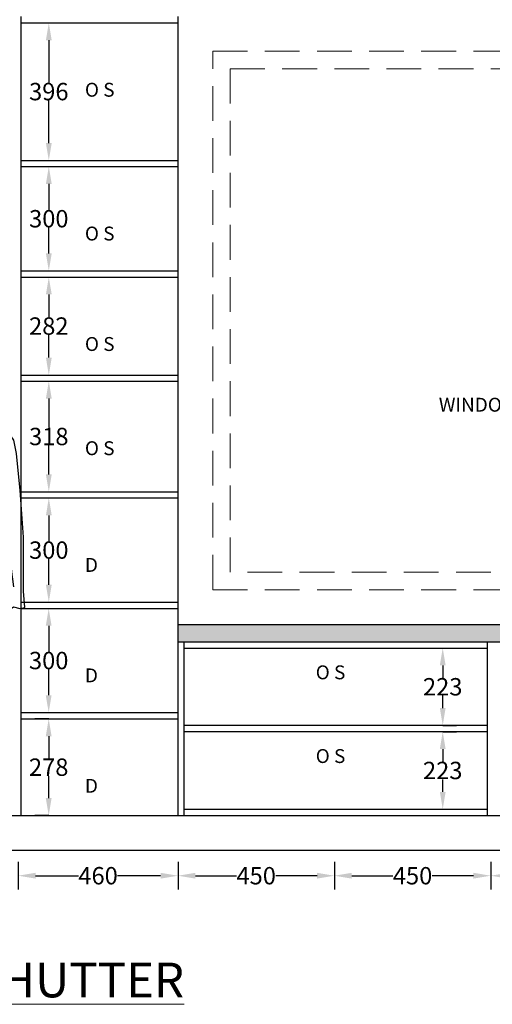
# Model space of a CAD drawing. Units: millimetres. Extents: x -472 to 16192, y -4730 to 4331.
# Tile 6 of 8: x 12774 to 14134, y -4730 to -1895. Entities that reach past the tile are written whole.
import ezdxf

# ---------------------------------------------------------------- set-up
doc = ezdxf.new("R2010")
doc.units = ezdxf.units.MM
doc.header["$MEASUREMENT"] = 0
doc.linetypes.add('DASHED', pattern=[0.75, 0.5, -0.25])
for name, color, linetype, lineweight in [('A-ANNO-DIMS', 2, 'Continuous', 18), ('A-ANNO-TEXT', 6, 'Continuous', 18), ('A-ELEV', 7, 'Continuous', 25), ('A-FURN', 8, 'Continuous', 25), ('A-GLAZ', 4, 'DASHED', 18)]:
    doc.layers.add(name, color=color, linetype=linetype, lineweight=lineweight)
doc.styles.get("Standard").update_dxf_attribs({"font": 'arial.ttf'})
doc.dimstyles.get("Standard").update_dxf_attribs({"dimtxt": 50, "dimasz": 50, "dimexe": 40, "dimexo": 40, "dimgap": 0.09, "dimtad": 0, "dimtih": 1, "dimtoh": 1, "dimdec": 0, "dimzin": 0, "dimdsep": 46, "dimtxsty": 'Standard', "dimcen": 0.09, "dimclrd": 1, "dimclre": 3, "dimclrt": 6, "dimadec": 0, "dimazin": 0, "dimtfac": 1, "dimtdec": 0, "dimtofl": 0, "dimtmove": 0, "dimatfit": 3, "dimfxl": 40, "dimfxlon": 1, "dimtolj": 1, "dimtzin": 0, "dimarcsym": 0})

# ---------------------------------------------------------------- blocks, each defined once
blk = doc.blocks.new('*D58')
at = {"layer": 'A-ANNO-DIMS', "color": 0, "lineweight": -2, "transparency": 16777216}
for p, q in [((12769.7, -4319.4), (12769.7, -4399.4)), ((13229.7, -4319.4), (13229.7, -4399.4)), ((12819.7, -4359.4), (12943.4, -4359.4)), ((13179.7, -4359.4), (13055.9, -4359.4))]:
    blk.add_line(p, q, dxfattribs=at)
at = {"layer": 'A-ANNO-DIMS', "color": 0, "transparency": 16777216}
for points in [[(12819.7, -4351), (12819.7, -4367.7), (12769.7, -4359.4)], [(13179.7, -4351), (13179.7, -4367.7), (13229.7, -4359.4)]]:
    blk.add_solid(points, dxfattribs=at)
at = {"layer": 'Defpoints', "color": 0, "transparency": 16777216}
for p in [(12769.7, -4185.9), (13229.7, -4185.9), (13229.7, -4359.4)]:
    blk.add_point(p, dxfattribs=at)
at = {"layer": 'A-ANNO-DIMS', "color": 0, "transparency": 16777216, "insert": (12999.7, -4359.4), "char_height": 50, "attachment_point": 5}
blk.add_mtext('\\A1;460', dxfattribs=at)
blk = doc.blocks.new('*D59')
at = {"layer": 'A-ANNO-DIMS', "color": 0, "lineweight": -2, "transparency": 16777216}
for p, q in [((13229.7, -4319.4), (13229.7, -4399.4)), ((13679.7, -4319.4), (13679.7, -4399.4)), ((13279.7, -4359.4), (13398.4, -4359.4)), ((13629.7, -4359.4), (13510.9, -4359.4))]:
    blk.add_line(p, q, dxfattribs=at)
at = {"layer": 'A-ANNO-DIMS', "color": 0, "transparency": 16777216}
for points in [[(13279.7, -4351), (13279.7, -4367.7), (13229.7, -4359.4)], [(13629.7, -4351), (13629.7, -4367.7), (13679.7, -4359.4)]]:
    blk.add_solid(points, dxfattribs=at)
at = {"layer": 'Defpoints', "color": 0, "transparency": 16777216}
for p in [(13229.7, -4185.9), (13679.7, -4185.9), (13679.7, -4359.4)]:
    blk.add_point(p, dxfattribs=at)
at = {"layer": 'A-ANNO-DIMS', "color": 0, "transparency": 16777216, "insert": (13454.7, -4359.4), "char_height": 50, "attachment_point": 5}
blk.add_mtext('\\A1;450', dxfattribs=at)
blk = doc.blocks.new('*D60')
at = {"layer": 'A-ANNO-DIMS', "color": 0, "lineweight": -2, "transparency": 16777216}
for p, q in [((13679.7, -4319.4), (13679.7, -4399.4)), ((14129.7, -4319.4), (14129.7, -4399.4)), ((13729.7, -4359.4), (13848.4, -4359.4)), ((14079.7, -4359.4), (13960.9, -4359.4))]:
    blk.add_line(p, q, dxfattribs=at)
at = {"layer": 'A-ANNO-DIMS', "color": 0, "transparency": 16777216}
for points in [[(13729.7, -4351), (13729.7, -4367.7), (13679.7, -4359.4)], [(14079.7, -4351), (14079.7, -4367.7), (14129.7, -4359.4)]]:
    blk.add_solid(points, dxfattribs=at)
at = {"layer": 'Defpoints', "color": 0, "transparency": 16777216}
for p in [(13679.7, -4185.9), (14129.7, -4185.9), (14129.7, -4359.4)]:
    blk.add_point(p, dxfattribs=at)
at = {"layer": 'A-ANNO-DIMS', "color": 0, "transparency": 16777216, "insert": (13904.7, -4359.4), "char_height": 50, "attachment_point": 5}
blk.add_mtext('\\A1;450', dxfattribs=at)
blk = doc.blocks.new('*D61')
at = {"layer": 'A-ANNO-DIMS', "color": 0, "lineweight": -2, "transparency": 16777216}
for p, q in [((14129.7, -4319.4), (14129.7, -4399.4)), ((14579.7, -4319.4), (14579.7, -4399.4)), ((14179.7, -4359.4), (14298.4, -4359.4)), ((14529.7, -4359.4), (14410.9, -4359.4))]:
    blk.add_line(p, q, dxfattribs=at)
at = {"layer": 'A-ANNO-DIMS', "color": 0, "transparency": 16777216}
for points in [[(14179.7, -4351), (14179.7, -4367.7), (14129.7, -4359.4)], [(14529.7, -4351), (14529.7, -4367.7), (14579.7, -4359.4)]]:
    blk.add_solid(points, dxfattribs=at)
at = {"layer": 'Defpoints', "color": 0, "transparency": 16777216}
for p in [(14129.7, -4185.9), (14579.7, -4185.9), (14579.7, -4359.4)]:
    blk.add_point(p, dxfattribs=at)
at = {"layer": 'A-ANNO-DIMS', "color": 0, "transparency": 16777216, "insert": (14354.7, -4359.4), "char_height": 50, "attachment_point": 5}
blk.add_mtext('\\A1;450', dxfattribs=at)
blk = doc.blocks.new('*D75')
at = {"layer": 'A-ANNO-DIMS', "color": 0, "lineweight": -2, "transparency": 16777216}
for p, q in [((12857.6, -3907.9), (12817.6, -3907.9)), ((12857.6, -3957.9), (12857.6, -4021.3)), ((12857.6, -4135.9), (12857.6, -4072.5)), ((12857.6, -4185.9), (12817.6, -4185.9))]:
    blk.add_line(p, q, dxfattribs=at)
at = {"layer": 'A-ANNO-DIMS', "color": 0, "transparency": 16777216}
for points in [[(12849.2, -3957.9), (12865.9, -3957.9), (12857.6, -3907.9)], [(12849.2, -4135.9), (12865.9, -4135.9), (12857.6, -4185.9)]]:
    blk.add_solid(points, dxfattribs=at)
at = {"layer": 'Defpoints', "color": 0, "transparency": 16777216}
for p in [(12857.6, -3907.9), (12886.2, -3907.9), (12886.2, -4185.9)]:
    blk.add_point(p, dxfattribs=at)
at = {"layer": 'A-ANNO-DIMS', "color": 0, "transparency": 16777216, "insert": (12857.6, -4046.9), "char_height": 50, "attachment_point": 5}
blk.add_mtext('\\A1;278', dxfattribs=at)
blk = doc.blocks.new('*D76')
at = {"layer": 'A-ANNO-DIMS', "color": 0, "lineweight": -2, "transparency": 16777216}
for p, q in [((12857.6, -3589.9), (12897.6, -3589.9)), ((12857.6, -3639.9), (12857.6, -3714.3)), ((12857.6, -3839.9), (12857.6, -3765.5)), ((12857.6, -3889.9), (12897.6, -3889.9))]:
    blk.add_line(p, q, dxfattribs=at)
at = {"layer": 'A-ANNO-DIMS', "color": 0, "transparency": 16777216}
for points in [[(12849.2, -3639.9), (12865.9, -3639.9), (12857.6, -3589.9)], [(12849.2, -3839.9), (12865.9, -3839.9), (12857.6, -3889.9)]]:
    blk.add_solid(points, dxfattribs=at)
at = {"layer": 'Defpoints', "color": 0, "transparency": 16777216}
for p in [(12857.6, -3589.9), (12857.6, -3589.9), (12857.6, -3889.9)]:
    blk.add_point(p, dxfattribs=at)
at = {"layer": 'A-ANNO-DIMS', "color": 0, "transparency": 16777216, "insert": (12857.6, -3739.9), "char_height": 50, "attachment_point": 5}
blk.add_mtext('\\A1;300', dxfattribs=at)
blk = doc.blocks.new('*D77')
at = {"layer": 'A-ANNO-DIMS', "color": 0, "lineweight": -2, "transparency": 16777216}
for p, q in [((12857.9, -3271.9), (12897.9, -3271.9)), ((12857.9, -3321.9), (12857.9, -3396.3)), ((12857.9, -3521.9), (12857.9, -3447.5)), ((12857.9, -3571.9), (12897.9, -3571.9))]:
    blk.add_line(p, q, dxfattribs=at)
at = {"layer": 'A-ANNO-DIMS', "color": 0, "transparency": 16777216}
for points in [[(12849.6, -3321.9), (12866.3, -3321.9), (12857.9, -3271.9)], [(12849.6, -3521.9), (12866.3, -3521.9), (12857.9, -3571.9)]]:
    blk.add_solid(points, dxfattribs=at)
at = {"layer": 'Defpoints', "color": 0, "transparency": 16777216}
for p in [(12857.9, -3271.9), (12857.9, -3271.9), (12857.9, -3571.9)]:
    blk.add_point(p, dxfattribs=at)
at = {"layer": 'A-ANNO-DIMS', "color": 0, "transparency": 16777216, "insert": (12857.9, -3421.9), "char_height": 50, "attachment_point": 5}
blk.add_mtext('\\A1;300', dxfattribs=at)
blk = doc.blocks.new('*D78')
at = {"layer": 'A-ANNO-DIMS', "color": 0, "lineweight": -2, "transparency": 16777216}
for p, q in [((12857.9, -2935.9), (12897.9, -2935.9)), ((12857.9, -2985.9), (12857.9, -3069.3)), ((12857.9, -3203.9), (12857.9, -3120.5)), ((12857.9, -3253.9), (12897.9, -3253.9))]:
    blk.add_line(p, q, dxfattribs=at)
at = {"layer": 'A-ANNO-DIMS', "color": 0, "transparency": 16777216}
for points in [[(12849.6, -2985.9), (12866.3, -2985.9), (12857.9, -2935.9)], [(12849.6, -3203.9), (12866.3, -3203.9), (12857.9, -3253.9)]]:
    blk.add_solid(points, dxfattribs=at)
at = {"layer": 'Defpoints', "color": 0, "transparency": 16777216}
for p in [(12857.9, -2935.9), (12857.9, -2935.9), (12857.9, -3253.9)]:
    blk.add_point(p, dxfattribs=at)
at = {"layer": 'A-ANNO-DIMS', "color": 0, "transparency": 16777216, "insert": (12857.9, -3094.9), "char_height": 50, "attachment_point": 5}
blk.add_mtext('\\A1;318', dxfattribs=at)
blk = doc.blocks.new('*D79')
at = {"layer": 'A-ANNO-DIMS', "color": 0, "lineweight": -2, "transparency": 16777216}
for p, q in [((12857.9, -2635.9), (12897.9, -2635.9)), ((12857.9, -2685.9), (12857.9, -2751.3)), ((12857.9, -2867.9), (12857.9, -2802.5)), ((12857.9, -2917.9), (12897.9, -2917.9))]:
    blk.add_line(p, q, dxfattribs=at)
at = {"layer": 'A-ANNO-DIMS', "color": 0, "transparency": 16777216}
for points in [[(12849.6, -2685.9), (12866.3, -2685.9), (12857.9, -2635.9)], [(12849.6, -2867.9), (12866.3, -2867.9), (12857.9, -2917.9)]]:
    blk.add_solid(points, dxfattribs=at)
at = {"layer": 'Defpoints', "color": 0, "transparency": 16777216}
for p in [(12857.9, -2635.9), (12857.9, -2635.9), (12857.9, -2917.9)]:
    blk.add_point(p, dxfattribs=at)
at = {"layer": 'A-ANNO-DIMS', "color": 0, "transparency": 16777216, "insert": (12857.9, -2776.9), "char_height": 50, "attachment_point": 5}
blk.add_mtext('\\A1;282', dxfattribs=at)
blk = doc.blocks.new('*D80')
at = {"layer": 'A-ANNO-DIMS', "color": 0, "lineweight": -2, "transparency": 16777216}
for p, q in [((12857.9, -2317.9), (12897.9, -2317.9)), ((12857.9, -2367.9), (12857.9, -2442.3)), ((12857.9, -2567.9), (12857.9, -2493.5)), ((12857.9, -2617.9), (12897.9, -2617.9))]:
    blk.add_line(p, q, dxfattribs=at)
at = {"layer": 'A-ANNO-DIMS', "color": 0, "transparency": 16777216}
for points in [[(12849.6, -2367.9), (12866.3, -2367.9), (12857.9, -2317.9)], [(12849.6, -2567.9), (12866.3, -2567.9), (12857.9, -2617.9)]]:
    blk.add_solid(points, dxfattribs=at)
at = {"layer": 'Defpoints', "color": 0, "transparency": 16777216}
for p in [(12857.9, -2317.9), (12857.9, -2317.9), (12857.9, -2617.9)]:
    blk.add_point(p, dxfattribs=at)
at = {"layer": 'A-ANNO-DIMS', "color": 0, "transparency": 16777216, "insert": (12857.9, -2467.9), "char_height": 50, "attachment_point": 5}
blk.add_mtext('\\A1;300', dxfattribs=at)
blk = doc.blocks.new('*D81')
at = {"layer": 'A-ANNO-DIMS', "color": 0, "lineweight": -2, "transparency": 16777216}
for p, q in [((12857.9, -1903.9), (12897.9, -1903.9)), ((12857.9, -1953.9), (12857.9, -2076.3)), ((12857.9, -2249.9), (12857.9, -2127.5)), ((12857.9, -2299.9), (12897.9, -2299.9))]:
    blk.add_line(p, q, dxfattribs=at)
at = {"layer": 'A-ANNO-DIMS', "color": 0, "transparency": 16777216}
for points in [[(12849.6, -1953.9), (12866.3, -1953.9), (12857.9, -1903.9)], [(12849.6, -2249.9), (12866.3, -2249.9), (12857.9, -2299.9)]]:
    blk.add_solid(points, dxfattribs=at)
at = {"layer": 'Defpoints', "color": 0, "transparency": 16777216}
for p in [(12857.9, -1903.9), (12857.9, -1903.9), (12857.9, -2299.9)]:
    blk.add_point(p, dxfattribs=at)
at = {"layer": 'A-ANNO-DIMS', "color": 0, "transparency": 16777216, "insert": (12857.9, -2101.9), "char_height": 50, "attachment_point": 5}
blk.add_mtext('\\A1;396', dxfattribs=at)
blk = doc.blocks.new('*D86')
at = {"layer": 'A-ANNO-DIMS', "color": 0, "lineweight": -2, "transparency": 16777216}
for p, q in [((11734.7, -2935.9), (11774.7, -2935.9)), ((11734.7, -2985.9), (11734.7, -3526.3)), ((11734.7, -4117.9), (11734.7, -3577.5)), ((11774.7, -4167.9), (11694.7, -4167.9))]:
    blk.add_line(p, q, dxfattribs=at)
at = {"layer": 'A-ANNO-DIMS', "color": 0, "transparency": 16777216}
for points in [[(11726.4, -2985.9), (11743, -2985.9), (11734.7, -2935.9)], [(11726.4, -4117.9), (11743, -4117.9), (11734.7, -4167.9)]]:
    blk.add_solid(points, dxfattribs=at)
at = {"layer": 'Defpoints', "color": 0, "transparency": 16777216}
for p in [(11734.7, -2935.9), (11734.7, -4167.9), (14004.4, -4167.9)]:
    blk.add_point(p, dxfattribs=at)
at = {"layer": 'A-ANNO-DIMS', "color": 0, "transparency": 16777216, "insert": (11734.7, -3551.9), "char_height": 50, "attachment_point": 5}
blk.add_mtext('\\A1;1232', dxfattribs=at)
blk = doc.blocks.new('*D87')
at = {"layer": 'A-ANNO-DIMS', "color": 0, "lineweight": -2, "transparency": 16777216}
for p, q in [((11774.7, -3944.9), (11694.7, -3944.9)), ((11734.7, -3994.9), (11734.7, -4030.8)), ((11734.7, -4117.9), (11734.7, -4082)), ((11774.7, -4167.9), (11694.7, -4167.9))]:
    blk.add_line(p, q, dxfattribs=at)
at = {"layer": 'A-ANNO-DIMS', "color": 0, "transparency": 16777216}
for points in [[(11726.4, -3994.9), (11743, -3994.9), (11734.7, -3944.9)], [(11726.4, -4117.9), (11743, -4117.9), (11734.7, -4167.9)]]:
    blk.add_solid(points, dxfattribs=at)
at = {"layer": 'Defpoints', "color": 0, "transparency": 16777216}
for p in [(11734.7, -3944.9), (13999.1, -3944.9), (14004.4, -4167.9)]:
    blk.add_point(p, dxfattribs=at)
at = {"layer": 'A-ANNO-DIMS', "color": 0, "transparency": 16777216, "insert": (11734.7, -4056.4), "char_height": 50, "attachment_point": 5}
blk.add_mtext('\\A1;223', dxfattribs=at)
blk = doc.blocks.new('*D88')
at = {"layer": 'A-ANNO-DIMS', "color": 0, "lineweight": -2, "transparency": 16777216}
for p, q in [((13991.5, -3944.9), (14031.5, -3944.9)), ((13991.5, -3994.9), (13991.5, -4030.8)), ((13991.5, -4117.9), (13991.5, -4082)), ((13991.5, -4167.9), (14031.5, -4167.9))]:
    blk.add_line(p, q, dxfattribs=at)
at = {"layer": 'A-ANNO-DIMS', "color": 0, "transparency": 16777216}
for points in [[(13983.2, -3994.9), (13999.8, -3994.9), (13991.5, -3944.9)], [(13983.2, -4117.9), (13999.8, -4117.9), (13991.5, -4167.9)]]:
    blk.add_solid(points, dxfattribs=at)
at = {"layer": 'Defpoints', "color": 0, "transparency": 16777216}
for p in [(13973.3, -3944.9), (13991.5, -3944.9), (13973.3, -4167.9)]:
    blk.add_point(p, dxfattribs=at)
at = {"layer": 'A-ANNO-DIMS', "color": 0, "transparency": 16777216, "insert": (13991.5, -4056.4), "char_height": 50, "attachment_point": 5}
blk.add_mtext('\\A1;223', dxfattribs=at)
blk = doc.blocks.new('*D89')
at = {"layer": 'A-ANNO-DIMS', "color": 0, "lineweight": -2, "transparency": 16777216}
for p, q in [((13991.5, -3703.9), (14031.5, -3703.9)), ((13991.5, -3753.9), (13991.5, -3789.8)), ((13991.5, -3876.9), (13991.5, -3841)), ((13991.5, -3926.9), (14031.5, -3926.9))]:
    blk.add_line(p, q, dxfattribs=at)
at = {"layer": 'A-ANNO-DIMS', "color": 0, "transparency": 16777216}
for points in [[(13983.2, -3753.9), (13999.8, -3753.9), (13991.5, -3703.9)], [(13983.2, -3876.9), (13999.8, -3876.9), (13991.5, -3926.9)]]:
    blk.add_solid(points, dxfattribs=at)
at = {"layer": 'Defpoints', "color": 0, "transparency": 16777216}
for p in [(13991.5, -3703.9), (13991.5, -3703.9), (13991.5, -3926.9)]:
    blk.add_point(p, dxfattribs=at)
at = {"layer": 'A-ANNO-DIMS', "color": 0, "transparency": 16777216, "insert": (13991.5, -3815.4), "char_height": 50, "attachment_point": 5}
blk.add_mtext('\\A1;223', dxfattribs=at)
blk = doc.blocks.new('7')
for p, q in [((3901.77, 12903.37), (3898.37, 12903.37)), ((3898.37, 12903.37), (3898.37, 12902.56)), ((3901.6, 12902.56), (3898.37, 12902.56)), ((3901.81, 12902.56), (3906.72, 12902.56)), ((3902.01, 12903.37), (3906.88, 12903.37)), ((3903.8, 12903.37), (3905.4, 12903.37)), ((3906.93, 12902.56), (3911.77, 12902.56)), ((3907.13, 12903.37), (3911.93, 12903.37)), ((3911.97, 12902.56), (3916.93, 12902.56)), ((3912.18, 12903.37), (3917.09, 12903.37)), ((3917.13, 12902.56), (3921.77, 12902.56)), ((3917.33, 12903.37), (3921.94, 12903.37)), ((3921.98, 12902.56), (3927.26, 12902.56)), ((3922.18, 12903.37), (3927.26, 12903.37)), ((3927.26, 12903.37), (3927.26, 12902.56)), ((3901.99, 12900.85), (3901.37, 12900)), ((3902.38, 12900.93), (3901.99, 12900.85)), ((3902.35, 12900.89), (3902.35, 12901.61)), ((3902.69, 12900.85), (3902.38, 12900.93)), ((3902.55, 12901.75), (3902.55, 12900.89)), ((3903.23, 12900.39), (3902.69, 12900.85)), ((3907.13, 12900.85), (3906.51, 12900)), ((3907.52, 12900.93), (3907.13, 12900.85)), ((3907.47, 12900.89), (3907.47, 12901.61)), ((3907.83, 12900.85), (3907.52, 12900.93)), ((3907.67, 12901.75), (3907.67, 12900.89)), ((3908.37, 12900.39), (3907.83, 12900.85)), ((3912.25, 12900.85), (3911.62, 12900)), ((3912.63, 12900.93), (3912.25, 12900.85)), ((3912.51, 12900.89), (3912.51, 12901.61)), ((3912.94, 12900.85), (3912.63, 12900.93)), ((3912.72, 12901.75), (3912.72, 12900.89)), ((3913.49, 12900.39), (3912.94, 12900.85)), ((3917.39, 12900.85), (3916.76, 12900)), ((3917.77, 12900.93), (3917.39, 12900.85)), ((3917.67, 12900.91), (3917.67, 12901.61)), ((3918.08, 12900.85), (3917.77, 12900.93)), ((3917.87, 12901.75), (3917.87, 12900.92)), ((3918.63, 12900.39), (3918.08, 12900.85)), ((3922.16, 12900.76), (3921.8, 12900.21)), ((3922.57, 12901.03), (3922.16, 12900.76)), ((3922.57, 12901.03), (3922.35, 12900.7)), ((3922.52, 12901), (3922.52, 12901.61)), ((3922.75, 12901), (3922.57, 12901.03)), ((3922.72, 12901.75), (3922.72, 12901.02)), ((3923.13, 12900.79), (3922.75, 12901)), ((3923.47, 12900.38), (3923.13, 12900.79)), ((3901.37, 12900), (3900.98, 12899.12)), ((3903.54, 12899.74), (3903.23, 12900.39)), ((3903.78, 12899.26), (3903.54, 12899.74)), ((3906.51, 12900), (3906.12, 12899.12)), ((3908.68, 12899.74), (3908.37, 12900.39)), ((3908.92, 12899.26), (3908.68, 12899.74)), ((3911.62, 12900), (3911.24, 12899.12)), ((3913.8, 12899.74), (3913.49, 12900.39)), ((3914.03, 12899.26), (3913.8, 12899.74)), ((3916.76, 12900), (3916.38, 12899.12)), ((3918.94, 12899.74), (3918.63, 12900.39)), ((3919.17, 12899.26), (3918.94, 12899.74)), ((3921.6, 12899.78), (3921.4, 12899.16)), ((3921.8, 12900.21), (3921.6, 12899.78)), ((3922.02, 12899.87), (3921.8, 12899.21)), ((3922.35, 12900.7), (3922.02, 12899.87)), ((3923.71, 12900.01), (3923.47, 12900.38)), ((3924, 12899.6), (3923.71, 12900.01)), ((3924.38, 12899.09), (3923.92, 12899.61)), ((3924, 12899.6), (3924.26, 12898.31)), ((3900.85, 12898.74), (3899.74, 12897.19)), ((3900.98, 12899.12), (3900.85, 12898.73)), ((3901.25, 12897.93), (3900.85, 12898.74)), ((3902.03, 12896.26), (3901.25, 12897.93)), ((3902.33, 12898.32), (3901.78, 12897.67)), ((3903.03, 12897.88), (3902.33, 12898.32)), ((3903.88, 12897.03), (3903.03, 12897.88)), ((3904.15, 12899.04), (3903.78, 12899.26)), ((3903.78, 12899.26), (3903.89, 12898.71)), ((3903.89, 12898.71), (3903.85, 12897.04)), ((3904.63, 12898.37), (3904.15, 12899.04)), ((3905.24, 12897.91), (3904.63, 12898.37)), ((3905.99, 12898.74), (3904.88, 12897.19)), ((3906.12, 12899.12), (3905.99, 12898.73)), ((3906.39, 12897.93), (3905.99, 12898.74)), ((3907.17, 12896.26), (3906.39, 12897.93)), ((3907.47, 12898.32), (3906.92, 12897.67)), ((3908.17, 12897.88), (3907.47, 12898.32)), ((3909.02, 12897.03), (3908.17, 12897.88)), ((3909.29, 12899.04), (3908.92, 12899.26)), ((3908.92, 12899.26), (3909.03, 12898.71)), ((3909.03, 12898.71), (3908.99, 12897.04)), ((3909.77, 12898.37), (3909.29, 12899.04)), ((3910.38, 12897.91), (3909.77, 12898.37)), ((3911.1, 12898.74), (3909.99, 12897.19)), ((3911.51, 12897.93), (3911.1, 12898.74)), ((3911.24, 12899.12), (3911.11, 12898.73)), ((3912.29, 12896.26), (3911.51, 12897.93)), ((3912.58, 12898.32), (3912.04, 12897.67)), ((3913.28, 12897.88), (3912.58, 12898.32)), ((3914.13, 12897.03), (3913.28, 12897.88)), ((3914.4, 12899.04), (3914.03, 12899.26)), ((3914.03, 12899.26), (3914.14, 12898.71)), ((3914.14, 12898.71), (3914.11, 12897.04)), ((3914.88, 12898.37), (3914.4, 12899.04)), ((3915.5, 12897.91), (3914.88, 12898.37)), ((3916.24, 12898.74), (3915.13, 12897.19)), ((3916.65, 12897.93), (3916.24, 12898.74)), ((3916.38, 12899.12), (3916.25, 12898.73)), ((3917.43, 12896.26), (3916.65, 12897.93)), ((3917.72, 12898.32), (3917.18, 12897.67)), ((3918.42, 12897.88), (3917.72, 12898.32)), ((3919.27, 12897.03), (3918.42, 12897.88)), ((3919.54, 12899.04), (3919.17, 12899.26)), ((3919.17, 12899.26), (3919.28, 12898.71)), ((3919.28, 12898.71), (3919.25, 12897.04)), ((3920.02, 12898.37), (3919.54, 12899.04)), ((3920.64, 12897.91), (3920.02, 12898.37)), ((3920.43, 12897.51), (3920.79, 12898.19)), ((3920.79, 12898.19), (3921.19, 12898.97)), ((3921.19, 12898.97), (3921.35, 12899.23)), ((3921.3, 12899.16), (3921.61, 12898.57)), ((3921.35, 12899.23), (3921.7, 12898.97)), ((3921.61, 12898.57), (3922.15, 12897.07)), ((3921.66, 12898.64), (3921.65, 12898.56)), ((3921.8, 12899.21), (3921.66, 12898.64)), ((3921.7, 12898.97), (3921.75, 12898.95)), ((3922.33, 12897.95), (3922.18, 12897.46)), ((3922.55, 12898.4), (3922.33, 12897.95)), ((3922.82, 12898.65), (3922.55, 12898.4)), ((3923.17, 12898.44), (3922.82, 12898.65)), ((3923.96, 12897.86), (3923.17, 12898.44)), ((3924.26, 12898.31), (3924.56, 12897.43)), ((3925.4, 12898.1), (3924.38, 12899.09)), ((3925.37, 12898.1), (3926.22, 12897.58)), ((3925.98, 12896.74), (3925.4, 12898.1)), ((3899.74, 12897.04), (3896.88, 12894.08)), ((3900.49, 12895.54), (3899.68, 12897.02)), ((3899.74, 12897.19), (3899.74, 12897.04)), ((3901.78, 12897.67), (3901.59, 12897.2)), ((3904.88, 12897.04), (3902.02, 12894.08)), ((3903.85, 12897.04), (3903.46, 12895.81)), ((3905.63, 12895.54), (3904.82, 12897.02)), ((3904.88, 12897.19), (3904.88, 12897.04)), ((3906.92, 12897.67), (3906.73, 12897.2)), ((3909.99, 12897.04), (3907.14, 12894.08)), ((3908.99, 12897.04), (3908.6, 12895.81)), ((3910.75, 12895.54), (3909.93, 12897.02)), ((3909.99, 12897.19), (3909.99, 12897.04)), ((3912.04, 12897.67), (3911.85, 12897.2)), ((3915.13, 12897.04), (3912.28, 12894.08)), ((3914.11, 12897.04), (3913.72, 12895.81)), ((3915.89, 12895.54), (3915.07, 12897.02)), ((3915.13, 12897.19), (3915.13, 12897.04)), ((3917.18, 12897.67), (3916.99, 12897.2)), ((3918.8, 12895.75), (3920.32, 12897.13)), ((3919.25, 12897.04), (3918.86, 12895.81)), ((3920.32, 12897.13), (3920.43, 12897.51)), ((3921.88, 12892.78), (3920.35, 12897.12)), ((3922.18, 12897.46), (3922.13, 12897.29)), ((3922.15, 12897.07), (3923.16, 12894.25)), ((3924.48, 12897.51), (3923.96, 12897.86)), ((3924.56, 12897.43), (3925.04, 12890.79)), ((3926.43, 12894.14), (3925.98, 12896.74)), ((3926.22, 12897.58), (3927.16, 12897.19)), ((3927.16, 12897.19), (3927.49, 12896.83)), ((3927.49, 12896.83), (3928.42, 12895.42)), ((3901.42, 12893.5), (3900.49, 12895.54)), ((3902.61, 12894.93), (3902.03, 12896.26)), ((3906.56, 12893.5), (3905.63, 12895.54)), ((3907.75, 12894.93), (3907.17, 12896.26)), ((3911.68, 12893.5), (3910.75, 12895.54)), ((3912.86, 12894.93), (3912.29, 12896.26)), ((3916.82, 12893.5), (3915.89, 12895.54)), ((3916.93, 12893.82), (3918.8, 12895.75)), ((3918, 12894.93), (3917.43, 12896.26)), ((3928.42, 12895.42), (3928.82, 12893.49)), ((3896.88, 12894.08), (3896.21, 12893.3)), ((3902.02, 12894.08), (3901.35, 12893.3)), ((3907.14, 12894.08), (3906.47, 12893.3)), ((3912.28, 12894.08), (3911.61, 12893.3)), ((3916.66, 12893.06), (3916.93, 12893.82)), ((3923.16, 12894.25), (3924.99, 12889.48)), ((3926.01, 12893.3), (3926.43, 12894.14)), ((3896.21, 12893.3), (3895.68, 12890.13)), ((3901.35, 12893.3), (3900.82, 12890.13)), ((3906.47, 12893.3), (3905.93, 12890.13)), ((3911.61, 12893.3), (3911.07, 12890.13)), ((3916.38, 12890.58), (3916.66, 12893.06)), ((3922.78, 12892.51), (3921.88, 12892.78)), ((3922.52, 12890.85), (3922.78, 12892.51)), ((3926.86, 12892.12), (3926.01, 12893.3)), ((3928.82, 12893.49), (3929.34, 12888.11)), ((3925.72, 12886.84), (3922.52, 12890.85)), ((3925.04, 12890.79), (3925.04, 12889.46)), ((3925.8, 12887.26), (3926.86, 12892.12)), ((3895.68, 12890.13), (3894.93, 12877.55)), ((3900.82, 12890.13), (3900.07, 12877.55)), ((3905.93, 12890.13), (3905.19, 12877.55)), ((3911.07, 12890.13), (3910.33, 12877.55)), ((3916.04, 12887.47), (3916.38, 12890.58)), ((3924.99, 12889.48), (3926.22, 12885.93)), ((3899.96, 12887.35), (3900.04, 12889.01)), ((3905.1, 12887.35), (3905.18, 12889.01)), ((3910.22, 12887.35), (3910.29, 12889.01)), ((3915.36, 12887.35), (3915.43, 12889.01)), ((3920.32, 12887.26), (3920.4, 12888.92)), ((3929.34, 12888.11), (3929.84, 12881.39)), ((3899.6, 12883.53), (3899.96, 12887.35)), ((3904.74, 12883.53), (3905.1, 12887.35)), ((3909.86, 12883.53), (3910.22, 12887.35)), ((3915, 12883.53), (3915.36, 12887.35)), ((3915.76, 12883.2), (3916.04, 12887.47)), ((3919.96, 12883.44), (3920.32, 12887.26)), ((3926.26, 12885.67), (3925.72, 12886.84)), ((3926.3, 12885.33), (3926.19, 12876.54)), ((3926.22, 12885.93), (3926.3, 12885.33)), ((3899.17, 12879.56), (3899.6, 12883.53)), ((3904.31, 12879.56), (3904.74, 12883.53)), ((3909.43, 12879.56), (3909.86, 12883.53)), ((3914.57, 12879.56), (3915, 12883.53)), ((3915.21, 12878.72), (3915.76, 12883.2)), ((3919.53, 12879.47), (3919.96, 12883.44)), ((3929.84, 12881.39), (3929.84, 12873.56)), ((3898.52, 12873.79), (3899.17, 12879.56)), ((3903.66, 12873.79), (3904.31, 12879.56)), ((3908.78, 12873.79), (3909.43, 12879.56)), ((3913.92, 12873.79), (3914.57, 12879.56)), ((3918.88, 12873.7), (3919.53, 12879.47)), ((3915, 12874.51), (3915.21, 12878.72)), ((3894.93, 12877.55), (3894.8, 12871.54)), ((3900.07, 12877.55), (3899.94, 12871.54)), ((3905.19, 12877.55), (3905.06, 12871.54)), ((3910.33, 12877.55), (3910.2, 12871.54)), ((3926.19, 12876.54), (3925.98, 12872.58)), ((3898.24, 12871.2), (3898.52, 12873.79)), ((3903.38, 12871.2), (3903.66, 12873.79)), ((3908.49, 12871.2), (3908.78, 12873.79)), ((3913.63, 12871.2), (3913.92, 12873.79)), ((3914.56, 12870.79), (3915, 12874.51)), ((3918.52, 12870.38), (3918.88, 12873.7)), ((3925.98, 12872.58), (3925.91, 12870.44)), ((3929.84, 12873.56), (3930.02, 12871.22)), ((3895.48, 12871.28), (3894.8, 12871.54)), ((3897.11, 12871.35), (3895.48, 12871.28)), ((3899.2, 12871.07), (3897.11, 12871.35)), ((3900.62, 12871.28), (3899.94, 12871.54)), ((3902.25, 12871.35), (3900.62, 12871.28)), ((3904.34, 12871.07), (3902.25, 12871.35)), ((3905.74, 12871.28), (3905.06, 12871.54)), ((3907.37, 12871.35), (3905.74, 12871.28)), ((3909.45, 12871.07), (3907.37, 12871.35)), ((3910.88, 12871.28), (3910.2, 12871.54)), ((3912.51, 12871.35), (3910.88, 12871.28)), ((3914.59, 12871.07), (3912.51, 12871.35)), ((3927.43, 12870.57), (3928.42, 12871.3)), ((3928.42, 12871.3), (3929.35, 12871.09)), ((3929.35, 12871.09), (3930.07, 12871.23)), ((3915.15, 12870.57), (3914.56, 12870.79)), ((3916.78, 12870.64), (3915.15, 12870.57)), ((3918.41, 12870.42), (3916.78, 12870.64)), ((3918.56, 12870.49), (3923.07, 12869.98)), ((3923.07, 12869.98), (3925.95, 12870.34)), ((3925.95, 12870.34), (3927.43, 12870.57))]:
    blk.add_line(p, q)
for centre, radius, start, end in [((3902.79, 12902.74), 1.19, 31.4138, 165.4823), ((3902.79, 12902.74), 0.991, 38.898, 165.4823), ((3907.9, 12902.74), 1.19, 31.4138, 165.4823), ((3907.9, 12902.74), 0.991, 38.898, 165.4823), ((3912.95, 12902.74), 1.19, 31.4138, 165.4823), ((3912.95, 12902.74), 0.991, 38.898, 165.4823), ((3918.11, 12902.74), 1.19, 31.4138, 165.4823), ((3918.11, 12902.74), 0.991, 38.898, 165.4823), ((3922.95, 12902.74), 1.19, 31.4138, 165.4823), ((3922.95, 12902.74), 0.991, 38.898, 165.4823), ((3902.81, 12902.74), 1.22, 165.4823, 247.8669), ((3902.81, 12902.74), 1.02, 165.4823, 255.3823), ((3902.7, 12902.33), 0.991, 354.9774, 12.9498), ((3903.79, 12902.23), 0.102, 171.8983, 358.0565), ((3902.7, 12902.33), 1.19, 354.9774, 10.7201), ((3907.93, 12902.74), 1.22, 165.4823, 247.8669), ((3907.93, 12902.74), 1.02, 165.4823, 255.3823), ((3907.81, 12902.33), 0.991, 354.9774, 12.9498), ((3908.9, 12902.23), 0.102, 171.8983, 358.0565), ((3907.81, 12902.33), 1.19, 354.9774, 10.7201), ((3912.97, 12902.74), 1.22, 165.4823, 247.8669), ((3912.97, 12902.74), 1.02, 165.4823, 255.3823), ((3912.86, 12902.33), 0.991, 354.9774, 12.9498), ((3913.95, 12902.23), 0.102, 171.8983, 358.0565), ((3912.86, 12902.33), 1.19, 354.9774, 10.7201), ((3918.13, 12902.74), 1.22, 165.4823, 247.8669), ((3918.13, 12902.74), 1.02, 165.4823, 255.3823), ((3918.02, 12902.33), 0.991, 354.9774, 12.9498), ((3919.11, 12902.23), 0.102, 171.8983, 358.0565), ((3918.02, 12902.33), 1.19, 354.9774, 10.7201), ((3922.98, 12902.74), 1.22, 165.4823, 247.8669), ((3922.98, 12902.74), 1.02, 165.4823, 255.3823), ((3922.87, 12902.33), 0.991, 354.9774, 12.9498), ((3923.95, 12902.23), 0.102, 171.8983, 358.0565), ((3922.87, 12902.33), 1.19, 354.9774, 10.7201), ((3897.26, 12891.85), 1.97, 15.7523, 111.1565), ((3902.4, 12891.85), 1.97, 15.7523, 111.1565), ((3907.51, 12891.85), 1.97, 15.7523, 111.1565), ((3912.65, 12891.85), 1.97, 15.7523, 111.1565), ((3917.62, 12891.76), 1.97, 15.7523, 111.1565), ((3890.5, 12887.86), 9.47, 359.9116, 24.988), ((3895.64, 12887.86), 9.47, 359.9116, 24.988), ((3900.76, 12887.86), 9.47, 359.9116, 24.988), ((3905.9, 12887.86), 9.47, 359.9116, 24.988), ((3910.86, 12887.76), 9.47, 359.9116, 24.988), ((4029.55, 12886.77), 101.91, 177.2767, 187.0811), ((3861.53, 12885.02), 36.92, 343.5409, 5.9886), ((3866.67, 12885.02), 36.92, 343.5409, 5.9886), ((3876.93, 12885.02), 36.92, 343.5409, 5.9886), ((3881.89, 12884.93), 36.92, 343.5409, 5.9886)]:
    blk.add_arc(centre, radius, start, end)
for centre in [(3925.62, 12884.08), (3925.62, 12878.91), (3925.62, 12873.74)]:
    blk.add_ellipse(centre, major_axis=(0, 0.503), ratio=0.580645)
blk = doc.blocks.new('*D100')
at = {"layer": 'A-ANNO-DIMS', "color": 1, "lineweight": -2, "transparency": 16777216}
for p, q in [((16116.7, -1835.9), (16116.7, -1785.9)), ((16116.7, -2035.9), (16116.7, -2085.9))]:
    blk.add_line(p, q, dxfattribs=at)
at = {"layer": 'A-ANNO-DIMS', "color": 3, "lineweight": -2, "transparency": 16777216}
for p, q in [((16076.7, -1885.9), (16156.7, -1885.9)), ((16076.7, -1985.9), (16156.7, -1985.9))]:
    blk.add_line(p, q, dxfattribs=at)
at = {"layer": 'A-ANNO-DIMS', "color": 1, "transparency": 16777216}
for points in [[(16108.3, -1835.9), (16125, -1835.9), (16116.7, -1885.9)], [(16108.3, -2035.9), (16125, -2035.9), (16116.7, -1985.9)]]:
    blk.add_solid(points, dxfattribs=at)
at = {"layer": 'Defpoints', "color": 0, "transparency": 16777216}
for p in [(5309, -1885.9), (5209, -1985.9), (16116.7, -1985.9)]:
    blk.add_point(p, dxfattribs=at)
at = {"layer": 'A-ANNO-DIMS', "color": 6, "transparency": 16777216, "insert": (16116.7, -1935.9), "char_height": 50, "attachment_point": 5}
blk.add_mtext('\\A1;100', dxfattribs=at)
blk = doc.blocks.new('*D101')
at = {"layer": 'A-ANNO-DIMS', "color": 3, "lineweight": -2, "transparency": 16777216}
for p, q in [((16076.7, -1985.9), (16156.7, -1985.9)), ((16076.7, -3535.9), (16156.7, -3535.9))]:
    blk.add_line(p, q, dxfattribs=at)
at = {"layer": 'A-ANNO-DIMS', "color": 1, "lineweight": -2, "transparency": 16777216}
for p, q in [((16116.7, -2035.9), (16116.7, -2735.3)), ((16116.7, -3485.9), (16116.7, -2786.5))]:
    blk.add_line(p, q, dxfattribs=at)
at = {"layer": 'A-ANNO-DIMS', "color": 1, "transparency": 16777216}
for points in [[(16108.3, -2035.9), (16125, -2035.9), (16116.7, -1985.9)], [(16108.3, -3485.9), (16125, -3485.9), (16116.7, -3535.9)]]:
    blk.add_solid(points, dxfattribs=at)
at = {"layer": 'Defpoints', "color": 0, "transparency": 16777216}
for p in [(5209, -1985.9), (5209, -3535.9), (16116.7, -3535.9)]:
    blk.add_point(p, dxfattribs=at)
at = {"layer": 'A-ANNO-DIMS', "color": 6, "transparency": 16777216, "insert": (16116.7, -2760.9), "char_height": 50, "attachment_point": 5}
blk.add_mtext('\\A1;1550', dxfattribs=at)
blk = doc.blocks.new('*D102')
at = {"layer": 'A-ANNO-DIMS', "color": 3, "lineweight": -2, "transparency": 16777216}
for p, q in [((16076.7, -2035.9), (16156.7, -2035.9)), ((16076.7, -3485.9), (16156.7, -3485.9))]:
    blk.add_line(p, q, dxfattribs=at)
at = {"layer": 'A-ANNO-DIMS', "color": 1, "lineweight": -2, "transparency": 16777216}
for p, q in [((16116.7, -2085.9), (16116.7, -2735.3)), ((16116.7, -3435.9), (16116.7, -2786.5))]:
    blk.add_line(p, q, dxfattribs=at)
at = {"layer": 'A-ANNO-DIMS', "color": 1, "transparency": 16777216}
for points in [[(16108.3, -2085.9), (16125, -2085.9), (16116.7, -2035.9)], [(16108.3, -3435.9), (16125, -3435.9), (16116.7, -3485.9)]]:
    blk.add_solid(points, dxfattribs=at)
at = {"layer": 'Defpoints', "color": 0, "transparency": 16777216}
for p in [(5159, -2035.9), (5159, -3485.9), (16116.7, -3485.9)]:
    blk.add_point(p, dxfattribs=at)
at = {"layer": 'A-ANNO-DIMS', "color": 6, "transparency": 16777216, "insert": (16116.7, -2760.9), "char_height": 50, "attachment_point": 5}
blk.add_mtext('\\A1;1450', dxfattribs=at)
blk = doc.blocks.new('*D103')
at = {"layer": 'A-ANNO-DIMS', "color": 1, "lineweight": -2, "transparency": 16777216}
for p, q in [((16116.7, -3485.9), (16116.7, -3435.9)), ((16116.7, -3685.9), (16116.7, -3735.9))]:
    blk.add_line(p, q, dxfattribs=at)
at = {"layer": 'A-ANNO-DIMS', "color": 3, "lineweight": -2, "transparency": 16777216}
for p, q in [((16076.7, -3535.9), (16156.7, -3535.9)), ((16076.7, -3635.9), (16156.7, -3635.9))]:
    blk.add_line(p, q, dxfattribs=at)
at = {"layer": 'A-ANNO-DIMS', "color": 1, "transparency": 16777216}
for points in [[(16108.3, -3485.9), (16125, -3485.9), (16116.7, -3535.9)], [(16108.3, -3685.9), (16125, -3685.9), (16116.7, -3635.9)]]:
    blk.add_solid(points, dxfattribs=at)
at = {"layer": 'Defpoints', "color": 0, "transparency": 16777216}
for p in [(5209, -3535.9), (5309, -3635.9), (16116.7, -3635.9)]:
    blk.add_point(p, dxfattribs=at)
at = {"layer": 'A-ANNO-DIMS', "color": 6, "transparency": 16777216, "insert": (16116.7, -3585.9), "char_height": 50, "attachment_point": 5}
blk.add_mtext('\\A1;100', dxfattribs=at)
blk = doc.blocks.new('*D104')
at = {"layer": 'A-ANNO-DIMS', "color": 1, "lineweight": -2, "transparency": 16777216}
for p, q in [((16116.7, -3585.9), (16116.7, -3535.9)), ((16116.7, -3735.9), (16116.7, -3785.9)), ((16116.7, -3785.9), (16066.7, -3785.9))]:
    blk.add_line(p, q, dxfattribs=at)
at = {"layer": 'A-ANNO-DIMS', "color": 3, "lineweight": -2, "transparency": 16777216}
for p, q in [((16076.7, -3635.9), (16156.7, -3635.9)), ((16076.7, -3685.9), (16156.7, -3685.9))]:
    blk.add_line(p, q, dxfattribs=at)
at = {"layer": 'A-ANNO-DIMS', "color": 1, "transparency": 16777216}
for points in [[(16108.3, -3585.9), (16125, -3585.9), (16116.7, -3635.9)], [(16108.3, -3735.9), (16125, -3735.9), (16116.7, -3685.9)]]:
    blk.add_solid(points, dxfattribs=at)
at = {"layer": 'Defpoints', "color": 0, "transparency": 16777216}
for p in [(5309, -3635.9), (5309, -3685.9), (16116.7, -3685.9)]:
    blk.add_point(p, dxfattribs=at)
at = {"layer": 'A-ANNO-DIMS', "color": 6, "transparency": 16777216, "insert": (16030.8, -3785.9), "char_height": 50, "attachment_point": 5}
blk.add_mtext('\\A1;50', dxfattribs=at)
blk = doc.blocks.new('*D106')
at = {"layer": 'A-ANNO-DIMS', "color": 3, "lineweight": -2, "transparency": 16777216}
for p, q in [((13329.7, -534.9), (13329.7, -454.9)), ((14929.7, -534.9), (14929.7, -454.9))]:
    blk.add_line(p, q, dxfattribs=at)
at = {"layer": 'A-ANNO-DIMS', "color": 1, "lineweight": -2, "transparency": 16777216}
for p, q in [((13379.7, -494.9), (14057.3, -494.9)), ((14879.7, -494.9), (14202, -494.9))]:
    blk.add_line(p, q, dxfattribs=at)
at = {"layer": 'A-ANNO-DIMS', "color": 1, "transparency": 16777216}
for points in [[(13379.7, -486.6), (13379.7, -503.2), (13329.7, -494.9)], [(14879.7, -486.6), (14879.7, -503.2), (14929.7, -494.9)]]:
    blk.add_solid(points, dxfattribs=at)
at = {"layer": 'Defpoints', "color": 0, "transparency": 16777216}
for p in [(14929.7, -494.9), (13329.7, -1985.9), (14929.7, -1985.9)]:
    blk.add_point(p, dxfattribs=at)
at = {"layer": 'A-ANNO-DIMS', "color": 6, "transparency": 16777216, "insert": (14129.7, -494.9), "char_height": 50, "attachment_point": 5}
blk.add_mtext('\\A1;1600', dxfattribs=at)
blk = doc.blocks.new('*D107')
at = {"layer": 'A-ANNO-DIMS', "color": 3, "lineweight": -2, "transparency": 16777216}
for p, q in [((13379.7, -534.9), (13379.7, -454.9)), ((14879.7, -534.9), (14879.7, -454.9))]:
    blk.add_line(p, q, dxfattribs=at)
at = {"layer": 'A-ANNO-DIMS', "color": 1, "lineweight": -2, "transparency": 16777216}
for p, q in [((13429.7, -494.9), (14057.3, -494.9)), ((14829.7, -494.9), (14202, -494.9))]:
    blk.add_line(p, q, dxfattribs=at)
at = {"layer": 'A-ANNO-DIMS', "color": 1, "transparency": 16777216}
for points in [[(13429.7, -486.6), (13429.7, -503.2), (13379.7, -494.9)], [(14829.7, -486.6), (14829.7, -503.2), (14879.7, -494.9)]]:
    blk.add_solid(points, dxfattribs=at)
at = {"layer": 'Defpoints', "color": 0, "transparency": 16777216}
for p in [(14879.7, -494.9), (13379.7, -2035.9), (14879.7, -2035.9)]:
    blk.add_point(p, dxfattribs=at)
at = {"layer": 'A-ANNO-DIMS', "color": 6, "transparency": 16777216, "insert": (14129.7, -494.9), "char_height": 50, "attachment_point": 5}
blk.add_mtext('\\A1;1500', dxfattribs=at)

msp = doc.modelspace()

# ---------------------------------------------------------------- hatches: boundary and pattern name
at = {"layer": 'A-GLAZ'}
h = msp.add_hatch(color=256, dxfattribs=at)
h.dxf.hatch_style = 1
h.paths.add_polyline_path([(15090.7, -3635.9), (13229.7, -3635.9), (13229.7, -3685.9), (15029.7, -3685.9), (15090.7, -3685.9)])

# ---------------------------------------------------------------- linework, layer by layer
at = {"layer": 'A-ELEV'}
for p, q in [((12778.7, -4185.9), (12778.7, -1885.9)), ((13229.7, -3685.9), (13229.7, -1885.9)), ((12778.7, -1903.9), (13229.7, -1903.9)), ((12778.7, -2299.9), (13229.7, -2299.9)), ((12778.7, -2317.9), (13229.7, -2317.9)), ((12778.7, -2617.9), (13229.7, -2617.9)), ((12778.7, -2635.9), (13229.7, -2635.9)), ((12778.7, -2917.9), (13229.7, -2917.9)), ((12778.7, -2935.9), (13229.7, -2935.9)), ((12778.7, -3253.9), (13229.7, -3253.9)), ((12778.7, -3271.9), (13229.7, -3271.9)), ((12778.7, -3571.9), (13229.7, -3571.9)), ((12778.7, -3589.9), (13229.7, -3589.9)), ((13229.7, -3635.9), (15090.7, -3635.9)), ((13229.7, -4185.9), (13229.7, -3685.9)), ((13229.7, -3685.9), (15090.7, -3685.9)), ((13247.7, -4185.9), (13247.7, -3685.9)), ((13247.7, -3703.9), (14120.7, -3703.9)), ((14120.7, -4185.9), (14120.7, -3685.9)), ((12778.7, -3889.9), (13229.7, -3889.9)), ((12778.7, -3907.9), (13229.7, -3907.9)), ((14120.7, -3926.9), (13247.7, -3926.9)), ((14120.7, -3944.9), (13247.7, -3944.9)), ((11840.7, -4185.9), (13229.7, -4185.9)), ((13229.7, -4185.9), (15090.7, -4185.9)), ((13247.7, -4167.9), (14120.7, -4167.9)), ((9720.7, -4285.9), (15320.7, -4285.9))]:
    msp.add_line(p, q, dxfattribs=at)
at = {"layer": 'A-GLAZ', "ltscale": 200}
for points in [[(13329.7, -1985.9), (14929.7, -1985.9), (14929.7, -3535.9), (13329.7, -3535.9)], [(13379.7, -2035.9), (14879.7, -2035.9), (14879.7, -3485.9), (13379.7, -3485.9)]]:
    msp.add_lwpolyline(points, close=True, dxfattribs=at)

# ---------------------------------------------------------------- block references
at = {"layer": 'A-FURN', "xscale": 19.91002939607444, "yscale": 19.91002939607444, "zscale": 19.91002939607444}
msp.add_blockref('7', (-65459, -259853.4), dxfattribs=at)

# ---------------------------------------------------------------- texts
at = {"layer": 'A-ANNO-TEXT', "attachment_point": 1}
for s, width, insert, char_height in [('O S', 327.678, (12961.8, -2076.6), 40), ('O S', 327.678, (12961.8, -2490.6), 40), ('O S', 327.678, (12961.8, -2808.6), 40), ('WINDOW', 327.678, (13980.3, -2983.4), 40), ('O S', 327.678, (12961.8, -3108.6), 40), ('D', 327.678, (12961.8, -3444.6), 40), ('D', 327.678, (12961.8, -3762.6), 40), ('O S', 327.678, (13626, -3753.9), 40), ('O S', 327.678, (13626, -3994.9), 40), ('D', 327.678, (12961.8, -4080.6), 40), ('{\\fArial|b1|i0|c0|p34;\\LELEVATION WITHOUT SHUTTER}', 3435.915, (11236.9, -4609.6), 100)]:
    msp.add_mtext_dynamic_manual_height_columns(s, width=width, gutter_width=1, heights=[0], dxfattribs=dict(at, insert=insert, char_height=char_height))

# ---------------------------------------------------------------- dimensions: what is measured, and where the dimension line sits
at = {"layer": 'A-ANNO-DIMS'}
for base, p1, p2, override, picture, middle in [((14929.7, -494.9), (13329.7, -1985.9), (14929.7, -1985.9), {"dimdec": 0, "dimlfac": 1, "dimrnd": 0, "dimzin": 0, "dimdsep": 46, "dimlunit": 2}, '*D106', (14129.7, -494.9)), ((14879.7, -494.9), (13379.7, -2035.9), (14879.7, -2035.9), {"dimdec": 0, "dimlfac": 1, "dimrnd": 0, "dimzin": 0, "dimdsep": 46, "dimlunit": 2}, '*D107', (14129.7, -494.9)), ((13229.7, -4359.4), (12769.7, -4185.9), (13229.7, -4185.9), {"dimclrd": 0, "dimclre": 0, "dimclrt": 0, "dimtmove": 1}, '*D58', (12999.7, -4359.4)), ((13679.7, -4359.4), (13229.7, -4185.9), (13679.7, -4185.9), {"dimclrd": 0, "dimclre": 0, "dimclrt": 0, "dimtmove": 1}, '*D59', (13454.7, -4359.4)), ((14129.7, -4359.4), (13679.7, -4185.9), (14129.7, -4185.9), {"dimclrd": 0, "dimclre": 0, "dimclrt": 0, "dimtmove": 1}, '*D60', (13904.7, -4359.4)), ((14579.7, -4359.4), (14129.7, -4185.9), (14579.7, -4185.9), {"dimclrd": 0, "dimclre": 0, "dimclrt": 0, "dimtmove": 1}, '*D61', (14354.7, -4359.4))]:
    dim = msp.add_linear_dim(base=base, p1=p1, p2=p2, dimstyle='Standard', override=override, dxfattribs=at)
    dim.commit()
    dim.dimension.update_dxf_attribs({"geometry": picture, "text_midpoint": middle})
for base, p1, p2, override, picture, middle in [((16116.7, -1985.9), (5309, -1885.9), (5209, -1985.9), {"dimdec": 0, "dimlfac": 1, "dimrnd": 0, "dimzin": 0, "dimdsep": 46, "dimlunit": 2}, '*D100', (16116.7, -1935.9)), ((12857.9, -1903.9), (12857.9, -2299.9), (12857.9, -1903.9), {"dimclrd": 0, "dimclre": 0, "dimclrt": 0}, '*D81', (12857.9, -2101.9)), ((16116.7, -3535.9), (5209, -1985.9), (5209, -3535.9), {"dimdec": 0, "dimlfac": 1, "dimrnd": 0, "dimzin": 0, "dimdsep": 46, "dimlunit": 2}, '*D101', (16116.7, -2760.9)), ((16116.7, -3485.9), (5159, -2035.9), (5159, -3485.9), {"dimdec": 0, "dimlfac": 1, "dimrnd": 0, "dimzin": 0, "dimdsep": 46, "dimlunit": 2}, '*D102', (16116.7, -2760.9)), ((12857.9, -2317.9), (12857.9, -2617.9), (12857.9, -2317.9), {"dimclrd": 0, "dimclre": 0, "dimclrt": 0}, '*D80', (12857.9, -2467.9)), ((12857.9, -2635.9), (12857.9, -2917.9), (12857.9, -2635.9), {"dimclrd": 0, "dimclre": 0, "dimclrt": 0}, '*D79', (12857.9, -2776.9)), ((11734.7, -4167.9), (11734.7, -2935.9), (14004.4, -4167.9), {"dimclrd": 0, "dimclre": 0, "dimclrt": 0, "dimtmove": 1}, '*D86', (11734.7, -3551.9)), ((12857.9, -2935.9), (12857.9, -3253.9), (12857.9, -2935.9), {"dimclrd": 0, "dimclre": 0, "dimclrt": 0}, '*D78', (12857.9, -3094.9)), ((12857.9, -3271.9), (12857.9, -3571.9), (12857.9, -3271.9), {"dimclrd": 0, "dimclre": 0, "dimclrt": 0}, '*D77', (12857.9, -3421.9)), ((16116.7, -3635.9), (5209, -3535.9), (5309, -3635.9), {"dimdec": 0, "dimlfac": 1, "dimrnd": 0, "dimzin": 0, "dimdsep": 46, "dimlunit": 2}, '*D103', (16116.7, -3585.9)), ((16116.7, -3685.9), (5309, -3635.9), (5309, -3685.9), {"dimdec": 0, "dimlfac": 1, "dimrnd": 0, "dimzin": 0, "dimdsep": 46, "dimlunit": 2}, '*D104', (16030.8, -3785.9)), ((12857.6, -3589.9), (12857.6, -3889.9), (12857.6, -3589.9), {"dimclrd": 0, "dimclre": 0, "dimclrt": 0}, '*D76', (12857.6, -3739.9)), ((13991.5, -3703.9), (13991.5, -3926.9), (13991.5, -3703.9), {"dimclrd": 0, "dimclre": 0, "dimclrt": 0}, '*D89', (13991.5, -3815.4)), ((12857.6, -3907.9), (12886.2, -4185.9), (12886.2, -3907.9), {"dimclrd": 0, "dimclre": 0, "dimclrt": 0}, '*D75', (12857.6, -4046.9)), ((11734.7, -3944.9), (14004.4, -4167.9), (13999.1, -3944.9), {"dimclrd": 0, "dimclre": 0, "dimclrt": 0, "dimtmove": 1}, '*D87', (11734.7, -4056.4)), ((13991.5, -3944.9), (13973.3, -4167.9), (13973.3, -3944.9), {"dimclrd": 0, "dimclre": 0, "dimclrt": 0}, '*D88', (13991.5, -4056.4))]:
    dim = msp.add_linear_dim(base=base, p1=p1, p2=p2, angle=90, dimstyle='Standard', override=override, dxfattribs=at)
    dim.commit()
    dim.dimension.update_dxf_attribs({"geometry": picture, "text_midpoint": middle})

doc.saveas('drawing.dxf')
